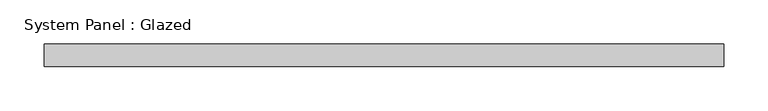
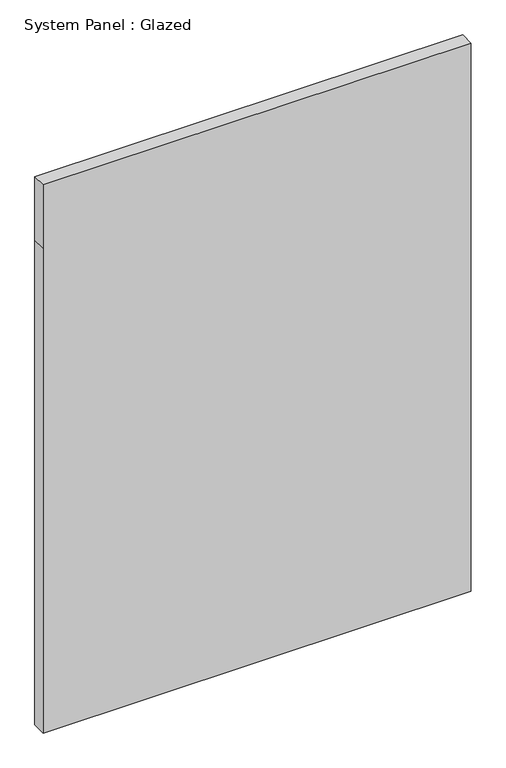
"""IFC4 building model written with IfcOpenShell, lengths in millimetres: plate geometry, System Panel : Glazed."""

from ifc_helpers import new_model, si_unit, frame, origin, place, context, project, spatial, polyline, outline, extrude, source, transform, mapped, element, save


def system_panel_glazed_4e21c323(model_context):
    return source(origin(), model_context, "Body", "SweptSolid", [
        extrude(outline(polyline([(0.0, -384.175), (0.0, 384.175), (919.5744987, 384.175), (1040.2244987, 384.175), (1040.2244987, -384.175), (919.5744987, -384.175), (0.0, -384.175)])), frame((0.0, 19.05, 0.0), z_axis=(0.0, 1.0, 0.0), x_axis=(0.0, 0.0, 1.0)), (0.0, 0.0, 1.0), 25.4),
    ])


if __name__ == "__main__":
    model = new_model("IFC4")
    model_context = context("Model", 3, world=origin())
    ifc_project = project(units=[si_unit("LENGTHUNIT", "METRE", prefix="MILLI")], contexts=[model_context])
    site = spatial("IfcSite", under=ifc_project)
    building = spatial("IfcBuilding", under=site)
    placement = place(None, origin())
    system_panel_glazed_shape = system_panel_glazed_4e21c323(model_context)
    element("IfcPlate", 1, ObjectType="System Panel : Glazed", at=placement, inside=building, context=model_context, shape_type="MappedRepresentation", body=[
        mapped(system_panel_glazed_shape, transform((0.0, 0.0, 0.0), x_axis=(1.0, 0.0, 0.0), y_axis=(0.0, 1.0, 0.0), z_axis=(0.0, 0.0, 1.0))),
    ])
    save(model, "model.ifc")

# Revit data of these elements
# Type "System Panel : Glazed"
#   Construction Type Id = "GSP4R"
#   Analytic Construction = "1/8 in Pilkington single glazing"
#   Visual Light Transmittance = 0.9
#   Solar Heat Gain Coefficient = 0.86
#   Heat Transfer Coefficient (U) = 1.18115 BTU/(h·ft²·°F)
#   Define Thermal Properties by = 1
# Element 1 (IfcPlate, "System Panel : Glazed")
#   Materials on its faces: "Glass"
# Materials
#   "Glass": class "Glass", colour RGB 0 128 192, transparency 0.75, Description = "Soda Lime Glass", Cost = 0
